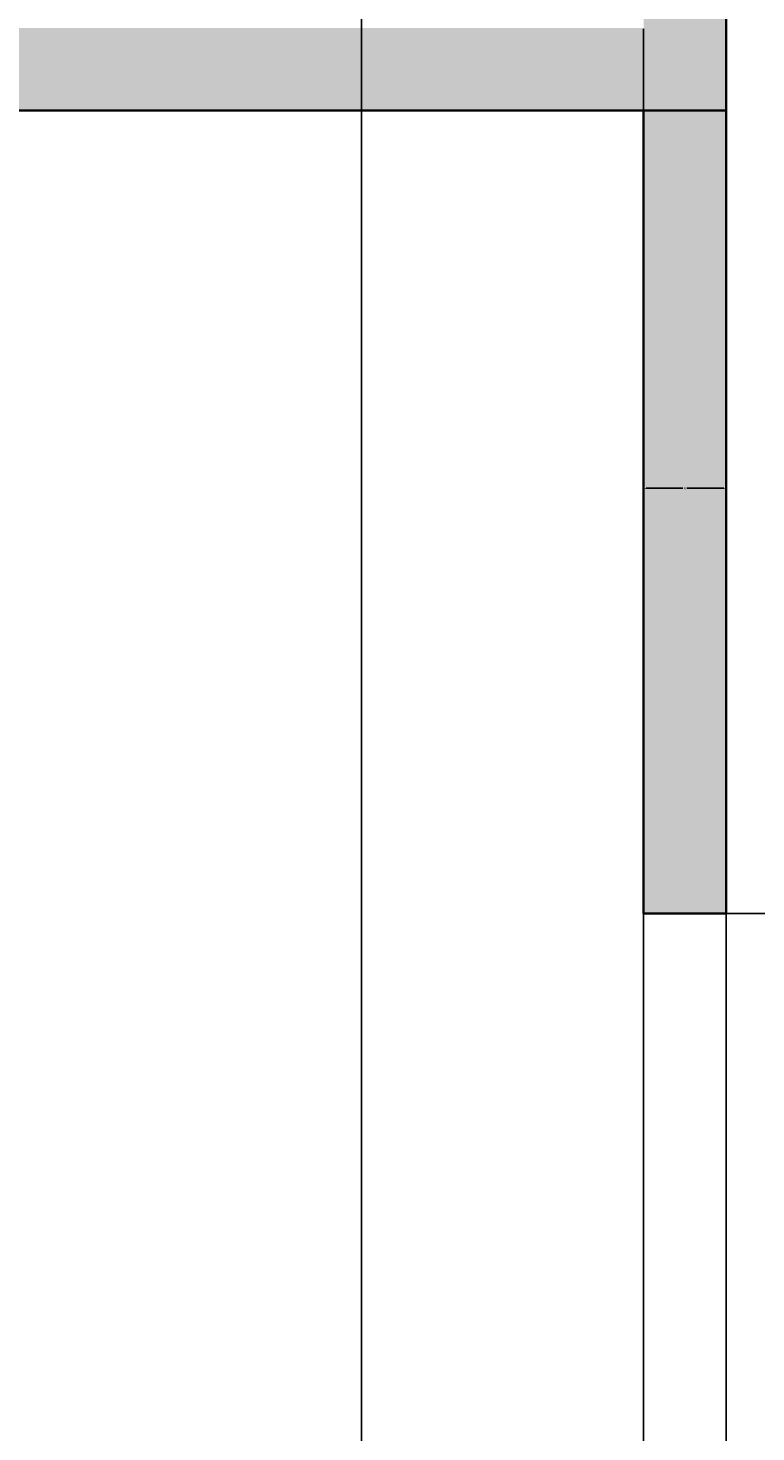
# Model space of a CAD drawing. Units: inches. Extents: x 2549 to 3108, y 1683 to 2362.
# Tile 16 of 30: x 2762 to 2815, y 1979 to 2081. Entities that reach past the tile are written whole.
import ezdxf

# ---------------------------------------------------------------- set-up
doc = ezdxf.new("R2010")
doc.units = ezdxf.units.IN
for name, color, linetype, lineweight in [('A-ANNO-DIMS', 2, 'Continuous', 18), ('A-WALL', 7, 'Continuous', 35), ('A-WALL-PATT', 89, 'Continuous', 13)]:
    doc.layers.add(name, color=color, linetype=linetype, lineweight=lineweight)
doc.layers.add('C-PKNG-VEHI-PATT', color=251, linetype='Continuous', lineweight=13, true_color=0x636466)
doc.layers.add('C-PVMT-PATT', color=9, linetype='Continuous', lineweight=13, true_color=0xc7c8ca)
doc.styles.get("Standard").update_dxf_attribs({"font": 'arial.ttf'})
doc.dimstyles.get("Standard").update_dxf_attribs({"dimtxt": 0.18, "dimasz": 0.18, "dimexe": 0.18, "dimexo": 0.0625, "dimgap": 0.09, "dimtad": 0, "dimtih": 1, "dimtoh": 1, "dimdec": 4, "dimzin": 0, "dimdsep": 46, "dimtxsty": 'Standard', "dimcen": 0.09, "dimadec": 0, "dimazin": 0, "dimtfac": 1, "dimtdec": 4, "dimtofl": 0, "dimtmove": 0, "dimatfit": 3, "dimfxl": 1, "dimtolj": 1, "dimtzin": 0, "dimarcsym": 0})

# ---------------------------------------------------------------- blocks, each defined once
blk = doc.blocks.new('*D43')
at = {"layer": 'A-ANNO-DIMS', "color": 0, "lineweight": -2, "transparency": 16777216}
for p, q in [((2734.64, 2080.46), (2734.64, 1683.44)), ((2806.64, 2080.46), (2806.64, 1683.44)), ((2734.82, 1683.62), (2770.43, 1683.62)), ((2806.46, 1683.62), (2770.86, 1683.62))]:
    blk.add_line(p, q, dxfattribs=at)
at = {"layer": 'A-ANNO-DIMS', "color": 0, "transparency": 16777216}
for points in [[(2734.82, 1683.65), (2734.82, 1683.59), (2734.64, 1683.62)], [(2806.46, 1683.65), (2806.46, 1683.59), (2806.64, 1683.62)]]:
    blk.add_solid(points, dxfattribs=at)
at = {"layer": 'Defpoints', "color": 0, "transparency": 16777216}
for p in [(2734.64, 2080.52), (2806.64, 2080.52), (2806.64, 1683.62)]:
    blk.add_point(p, dxfattribs=at)
at = {"layer": 'A-ANNO-DIMS', "color": 0, "transparency": 16777216, "insert": (2770.64, 1683.62), "char_height": 0.18, "attachment_point": 5}
blk.add_mtext('\\A1;72', dxfattribs=at)
blk = doc.blocks.new('*D44')
at = {"layer": 'A-ANNO-DIMS', "color": 0, "lineweight": -2, "transparency": 16777216}
for p, q in [((2662.64, 2040.99), (2662.64, 1683.44)), ((2806.64, 2016.13), (2806.64, 1683.44)), ((2662.82, 1683.62), (2734.36, 1683.62)), ((2806.46, 1683.62), (2734.92, 1683.62))]:
    blk.add_line(p, q, dxfattribs=at)
at = {"layer": 'A-ANNO-DIMS', "color": 0, "transparency": 16777216}
for points in [[(2662.82, 1683.65), (2662.82, 1683.59), (2662.64, 1683.62)], [(2806.46, 1683.65), (2806.46, 1683.59), (2806.64, 1683.62)]]:
    blk.add_solid(points, dxfattribs=at)
at = {"layer": 'Defpoints', "color": 0, "transparency": 16777216}
for p in [(2662.64, 2041.06), (2806.64, 2016.19), (2806.64, 1683.62)]:
    blk.add_point(p, dxfattribs=at)
at = {"layer": 'A-ANNO-DIMS', "color": 0, "transparency": 16777216, "insert": (2734.64, 1683.62), "char_height": 0.18, "attachment_point": 5}
blk.add_mtext('\\A1;144', dxfattribs=at)
blk = doc.blocks.new('*D46')
at = {"layer": 'A-ANNO-DIMS', "color": 0, "lineweight": -2, "transparency": 16777216}
for p, q in [((2812.64, 2140.46), (2812.64, 1683.44)), ((3034.64, 2134.46), (3034.64, 1683.44)), ((2812.82, 1683.62), (2923.35, 1683.62)), ((3034.46, 1683.62), (2923.93, 1683.62))]:
    blk.add_line(p, q, dxfattribs=at)
at = {"layer": 'A-ANNO-DIMS', "color": 0, "transparency": 16777216}
for points in [[(2812.82, 1683.65), (2812.82, 1683.59), (2812.64, 1683.62)], [(3034.46, 1683.65), (3034.46, 1683.59), (3034.64, 1683.62)]]:
    blk.add_solid(points, dxfattribs=at)
at = {"layer": 'Defpoints', "color": 0, "transparency": 16777216}
for p in [(2812.64, 2140.52), (3034.64, 2134.52), (3034.64, 1683.62)]:
    blk.add_point(p, dxfattribs=at)
at = {"layer": 'A-ANNO-DIMS', "color": 0, "transparency": 16777216, "insert": (2923.64, 1683.62), "char_height": 0.18, "attachment_point": 5}
blk.add_mtext('\\A1;222', dxfattribs=at)
blk = doc.blocks.new('*D47')
at = {"layer": 'A-ANNO-DIMS', "color": 0, "lineweight": -2, "transparency": 16777216}
for p, q in [((2806.64, 2016.25), (2806.64, 2047.27)), ((2812.64, 2016.25), (2812.64, 2047.27)), ((2806.82, 2047.09), (2809.49, 2047.09)), ((2812.46, 2047.09), (2809.79, 2047.09))]:
    blk.add_line(p, q, dxfattribs=at)
at = {"layer": 'A-ANNO-DIMS', "color": 0, "transparency": 16777216}
for points in [[(2806.82, 2047.12), (2806.82, 2047.06), (2806.64, 2047.09)], [(2812.46, 2047.12), (2812.46, 2047.06), (2812.64, 2047.09)]]:
    blk.add_solid(points, dxfattribs=at)
at = {"layer": 'Defpoints', "color": 0, "transparency": 16777216}
for p in [(2812.64, 2047.09), (2806.64, 2016.19), (2812.64, 2016.19)]:
    blk.add_point(p, dxfattribs=at)
at = {"layer": 'A-ANNO-DIMS', "color": 0, "transparency": 16777216, "insert": (2809.64, 2047.09), "char_height": 0.18, "attachment_point": 5}
blk.add_mtext('\\A1;6', dxfattribs=at)
blk = doc.blocks.new('*D48')
at = {"layer": 'A-ANNO-DIMS', "color": 0, "lineweight": -2, "transparency": 16777216}
for p, q in [((2812.71, 2016.19), (2843.72, 2016.19)), ((2843.54, 2016.01), (2843.54, 1981.04)), ((2843.54, 1945.7), (2843.54, 1980.68)), ((2812.71, 1945.52), (2843.72, 1945.52))]:
    blk.add_line(p, q, dxfattribs=at)
at = {"layer": 'A-ANNO-DIMS', "color": 0, "transparency": 16777216}
for points in [[(2843.51, 2016.01), (2843.57, 2016.01), (2843.54, 2016.19)], [(2843.51, 1945.7), (2843.57, 1945.7), (2843.54, 1945.52)]]:
    blk.add_solid(points, dxfattribs=at)
at = {"layer": 'Defpoints', "color": 0, "transparency": 16777216}
for p in [(2812.64, 2016.19), (2812.64, 1945.52), (2843.54, 1945.52)]:
    blk.add_point(p, dxfattribs=at)
at = {"layer": 'A-ANNO-DIMS', "color": 0, "transparency": 16777216, "insert": (2843.54, 1980.86), "char_height": 0.18, "attachment_point": 5}
blk.add_mtext('\\A1;70.67', dxfattribs=at)
blk = doc.blocks.new('*D52')
at = {"layer": 'A-ANNO-DIMS', "color": 0, "lineweight": -2, "transparency": 16777216}
for p, q in [((2812.64, 1891.59), (2812.64, 2362.32)), ((2872.64, 1891.59), (2872.64, 2362.32)), ((2812.82, 2362.14), (2842.42, 2362.14)), ((2872.46, 2362.14), (2842.86, 2362.14))]:
    blk.add_line(p, q, dxfattribs=at)
at = {"layer": 'A-ANNO-DIMS', "color": 0, "transparency": 16777216}
for points in [[(2812.82, 2362.17), (2812.82, 2362.11), (2812.64, 2362.14)], [(2872.46, 2362.17), (2872.46, 2362.11), (2872.64, 2362.14)]]:
    blk.add_solid(points, dxfattribs=at)
at = {"layer": 'Defpoints', "color": 0, "transparency": 16777216}
for p in [(2872.64, 2362.14), (2812.64, 1891.52), (2872.64, 1891.52)]:
    blk.add_point(p, dxfattribs=at)
at = {"layer": 'A-ANNO-DIMS', "color": 0, "transparency": 16777216, "insert": (2842.64, 2362.14), "char_height": 0.18, "attachment_point": 5}
blk.add_mtext('\\A1;60', dxfattribs=at)
blk = doc.blocks.new('*D59')
at = {"layer": 'A-ANNO-DIMS', "color": 0, "lineweight": -2, "transparency": 16777216}
for p, q in [((2680.98, 1761.59), (2680.98, 2362.32)), ((2786.16, 1761.59), (2786.16, 2362.32)), ((2681.16, 2362.14), (2733.11, 2362.14)), ((2785.98, 2362.14), (2734.02, 2362.14))]:
    blk.add_line(p, q, dxfattribs=at)
at = {"layer": 'A-ANNO-DIMS', "color": 0, "transparency": 16777216}
for points in [[(2681.16, 2362.17), (2681.16, 2362.11), (2680.98, 2362.14)], [(2785.98, 2362.17), (2785.98, 2362.11), (2786.16, 2362.14)]]:
    blk.add_solid(points, dxfattribs=at)
at = {"layer": 'Defpoints', "color": 0, "transparency": 16777216}
for p in [(2786.16, 2362.14), (2680.98, 1761.52), (2786.16, 1761.52)]:
    blk.add_point(p, dxfattribs=at)
at = {"layer": 'A-ANNO-DIMS', "color": 0, "transparency": 16777216, "insert": (2733.57, 2362.14), "char_height": 0.18, "attachment_point": 5}
blk.add_mtext('\\A1;105.18', dxfattribs=at)

msp = doc.modelspace()

# ---------------------------------------------------------------- hatches: boundary and pattern name
at = {"layer": 'A-WALL-PATT'}
h = msp.add_hatch(color=256, dxfattribs=at)
h.dxf.hatch_style = 1
h.paths.add_polyline_path([(2638.6427, 2272.5237), (3034.6427, 2272.5237), (3034.6427, 1936.5237), (3043.6427, 1936.5237), (3043.6427, 2281.5237), (2629.6427, 2281.5237), (2629.6427, 2074.5237), (2812.6427, 2074.5237), (2812.6427, 2140.5237), (2785.7177, 2140.5237), (2785.7177, 2134.5237), (2806.6427, 2134.5237), (2806.6427, 2080.5237), (2638.6427, 2080.5237)])
h.paths.add_polyline_path([(2638.6427, 1972.5237), (2662.6427, 1972.5237), (2662.6427, 2041.0557), (2653.6427, 2041.0557), (2653.6427, 1978.5237), (2629.6427, 1978.5237), (2629.6427, 1795.5237), (2662.6427, 1795.5237), (2881.6427, 1795.5237), (2881.6427, 1936.5237), (2965.9351, 1936.5237), (2965.9351, 1974.5439), (2959.9351, 1974.5439), (2959.9351, 1945.5237), (2881.6427, 1945.5237), (2872.6427, 1945.5237), (2872.6427, 1804.5237), (2662.6427, 1804.5237), (2638.6427, 1804.5237)])
h = msp.add_hatch(color=256, dxfattribs=at)
h.dxf.hatch_style = 1
h.paths.add_polyline_path([(2747.213, 2140.5237), (2638.6427, 2140.5237), (2638.6427, 2134.5237), (2747.213, 2134.5237)])
h.paths.add_polyline_path([(2734.6427, 2109.4935), (2728.6427, 2109.4935), (2728.6427, 2080.5237), (2734.6427, 2080.5237)])
h.paths.add_polyline_path([(2812.6427, 2074.5237), (2806.6427, 2074.5237), (2806.6427, 2016.1911), (2812.6427, 2016.1911)])
h.paths.add_polyline_path([(2812.6427, 1945.5237), (2806.6427, 1945.5237), (2806.6427, 1885.5237), (2872.6427, 1885.5237), (2872.6427, 1891.5237), (2812.6427, 1891.5237)])
h.paths.add_polyline_path([(2812.6427, 1855.9859), (2806.6427, 1855.9859), (2806.6427, 1804.5237), (2812.6427, 1804.5237)])
at = {"layer": 'C-PKNG-VEHI-PATT'}
h = msp.add_hatch(color=256, dxfattribs=at)
h.dxf.hatch_style = 1
edge = h.paths.add_edge_path()
edge.add_ellipse((2935.7258, 1791.964), major_axis=(-50.66, 0), ratio=0.84230387, start_angle=248.165046, end_angle=265.722579)
edge.add_line((2938.911, 1834.5507), (2925.8653, 1834.5507))
edge.add_ellipse((2929.0505, 1791.964), major_axis=(50.66, 0), ratio=0.84230387, start_angle=94.277421, end_angle=111.834954)
edge.add_line((2912.8508, 1832.3947), (2914.2044, 1822.2495))
edge.add_ellipse((2930.6538, 1783.1023), major_axis=(-49.3014, 0), ratio=0.84230387, start_angle=-85.12993, end_angle=-67.208085, ccw=False)
edge.add_line((2927.1247, 1824.5225), (2937.6516, 1824.5225))
edge.add_ellipse((2934.1225, 1783.1023), major_axis=(49.3014, 0), ratio=0.84230387, start_angle=67.208085, end_angle=85.12993, ccw=False)
edge.add_line((2950.5719, 1822.2495), (2951.9255, 1832.3947))
edge = h.paths.add_edge_path()
edge.add_ellipse((2903.4793, 1857.3351), major_axis=(-34.7979, 0), ratio=0.84230387, start_angle=180, end_angle=209.43857)
edge.add_ellipse((2961.297, 1857.3351), major_axis=(34.7979, 0), ratio=0.84230387, start_angle=150.56143, end_angle=180)
edge.add_line((2926.4991, 1857.3351), (2926.4991, 1843.7609))
edge.add_ellipse((2924.1251, 1844.3143), major_axis=(-0.2209, 3.9278), ratio=0.60383358, start_angle=89.002014, end_angle=253.657408, ccw=False)
edge.add_line((2921.7512, 1844.2222), (2921.7512, 1853.3975))
edge.add_line((2921.7512, 1853.3975), (2925.269, 1855.8484))
edge.add_ellipse((2925.4782, 1855.4931), major_axis=(0.4584, 0), ratio=0.84230387, start_angle=90, end_angle=134.480211, ccw=False)
edge.add_line((2925.4782, 1855.8792), (2926.4991, 1855.8792))
edge.add_line((2926.4991, 1855.8792), (2926.4991, 1857.3351))
edge.add_ellipse((2961.297, 1857.3351), major_axis=(34.7979, 0), ratio=0.84230387, start_angle=150.56143, end_angle=180, ccw=False)
edge.add_line((2932.3882, 1873.6501), (2932.3882, 1875.7801))
edge.add_ellipse((2932.3882, 1875.3939), major_axis=(0.4584, 0), ratio=0.84230387, start_angle=90, end_angle=127.93313)
edge.add_line((2932.1366, 1875.7167), (2928.5915, 1873.7564))
edge.add_ellipse((2899.9271, 2002.4692), major_axis=(155.4756, 0), ratio=0.84230387, start_angle=-80.743434, end_angle=-77.445067, ccw=False)
edge.add_ellipse((2949.4402, 1715.2151), major_axis=(-189.1422, 0), ratio=0.84230387, start_angle=-79.790461, end_angle=-77.555373)
edge.add_ellipse((3300.3614, 1852.5642), major_axis=(-386.1662, 0), ratio=0.84230387, start_angle=-2.863715, end_angle=2.198541)
edge.add_ellipse((2929.0505, 1792.5159), major_axis=(-55.6192, 0), ratio=0.84230387, start_angle=-85.917589, end_angle=-72.280047, ccw=False)
edge.add_line((2925.7129, 1839.2798), (2939.0634, 1839.2798))
edge.add_ellipse((2935.7258, 1792.5159), major_axis=(55.6192, 0), ratio=0.84230387, start_angle=72.280047, end_angle=85.917589, ccw=False)
edge.add_ellipse((2564.4149, 1852.5642), major_axis=(-386.1662, 0), ratio=0.84230387, start_angle=177.801459, end_angle=182.863715)
edge.add_ellipse((2915.3361, 1715.2151), major_axis=(189.1422, 0), ratio=0.84230387, start_angle=77.555373, end_angle=79.790461)
edge.add_ellipse((2964.8492, 2002.4692), major_axis=(-155.4756, 0), ratio=0.84230387, start_angle=77.445067, end_angle=80.743434, ccw=False)
edge.add_line((2936.1848, 1873.7564), (2932.6397, 1875.7167))
edge.add_ellipse((2932.3882, 1875.3939), major_axis=(0.4584, 0), ratio=0.84230387, start_angle=52.06687, end_angle=90)
edge.add_line((2932.3882, 1875.7801), (2932.3882, 1873.6501))
edge.add_ellipse((2903.4793, 1857.3351), major_axis=(-34.7979, 0), ratio=0.84230387, start_angle=180, end_angle=209.43857, ccw=False)
edge.add_line((2938.2772, 1857.3351), (2938.2772, 1855.8792))
edge.add_line((2938.2772, 1855.8792), (2939.4059, 1855.8792))
edge.add_ellipse((2939.2981, 1855.4931), major_axis=(-0.4584, 0), ratio=0.84230387, start_angle=225.519789, end_angle=270, ccw=False)
edge.add_line((2939.5903, 1855.7906), (2943.0251, 1853.3975))
edge.add_line((2943.0251, 1853.3975), (2943.0251, 1844.2222))
edge.add_ellipse((2940.6512, 1844.3143), major_axis=(0.2209, 3.9278), ratio=0.60383358, start_angle=106.342592, end_angle=270.997986, ccw=False)
edge.add_line((2938.2772, 1843.7609), (2938.2772, 1857.3351))
edge = h.paths.add_edge_path()
edge.add_ellipse((2932.3882, 1865.1973), major_axis=(91.081, 0), ratio=0.84230387, start_angle=256.401865, end_angle=283.598135, ccw=False)
edge.add_line((2914.2044, 1790.0239), (2914.2044, 1778.3622))
edge.add_ellipse((2932.3882, 1853.5356), major_axis=(91.081, 0), ratio=0.84230387, start_angle=256.401865, end_angle=283.598135)
edge.add_line((2950.5719, 1778.3622), (2950.5719, 1790.0239))
edge = h.paths.add_edge_path()
edge.add_ellipse((2948.7383, 1772.3145), major_axis=(1.8336, 0), ratio=0.84230387, start_angle=0, end_angle=90)
edge.add_line((2948.7383, 1773.859), (2916.038, 1773.859))
edge.add_ellipse((2916.038, 1772.3145), major_axis=(1.8336, 0), ratio=0.84230387, start_angle=90, end_angle=180)
edge.add_line((2914.2044, 1772.3145), (2914.2044, 1760.2558))
edge.add_line((2914.2044, 1760.2558), (2950.5719, 1760.2558))
edge.add_line((2950.5719, 1760.2558), (2950.5719, 1772.3145))
h.paths.add_polyline_path([(2748.8496, 2101.6383), (2798.148, 2101.6383), (2798.148, 2111.4248), (2748.8496, 2111.4248)], flags=9)
h.paths.add_polyline_path([(2685.2081, 2101.489), (2719.3253, 2101.489), (2719.3253, 2111.2819), (2685.2081, 2111.2819)], flags=9)
h.paths.add_polyline_path([(2814.6852, 1907.1328), (2847.8384, 1907.1328), (2847.8384, 1916.9258), (2814.6852, 1916.9258)], flags=9)
h.paths.add_polyline_path([(2814.3906, 1835.5864), (2848.0172, 1835.5864), (2848.0172, 1845.3794), (2814.3906, 1845.3794)], flags=9)
h.paths.add_polyline_path([(2800.5245, 1759.1674), (2853.7435, 1759.1674), (2853.7435, 1768.954), (2800.5245, 1768.954)], flags=9)
h.paths.add_polyline_path([(2972.4611, 1807.3305), (3015.3943, 1807.3305), (3015.3943, 1817.117), (2972.4611, 1817.117)], flags=9)
h.paths.add_polyline_path([(2902.3327, 1888.6731), (2937.9131, 1888.6731), (2937.9131, 1898.4661), (2902.3327, 1898.4661)], flags=9)
h.paths.add_polyline_path([(2712.1779, 1878.9039), (2754.1257, 1878.9039), (2754.1257, 1888.6904), (2712.1779, 1888.6904)], flags=9)
h.paths.add_polyline_path([(2614.0056, 2012.812), (2650.0251, 2012.812), (2650.0251, 2022.4371), (2614.0056, 2022.4371)], flags=9)
h.paths.add_polyline_path([(2713.3129, 2003.1645), (2747.4237, 2003.1645), (2747.4237, 2012.951), (2713.3129, 2012.951)], flags=9)
h.paths.add_polyline_path([(2950.1379, 2001.6934), (2982.2992, 2001.6934), (2982.2992, 2011.48), (2950.1379, 2011.48)], flags=9)
h.paths.add_polyline_path([(2940.864, 2238.5537), (2997.5066, 2238.5537), (2997.5066, 2248.3466), (2940.864, 2248.3466)], flags=9)
h.paths.add_polyline_path([(2821.5457, 2202.8348), (2855.663, 2202.8348), (2855.663, 2212.6278), (2821.5457, 2212.6278)], flags=9)
h.paths.add_polyline_path([(2661.8026, 2238.6249), (2718.4451, 2238.6249), (2718.4451, 2248.4179), (2661.8026, 2248.4179)], flags=9)
at = {"layer": 'C-PVMT-PATT'}
h = msp.add_hatch(color=256, dxfattribs=at)
h.dxf.hatch_style = 1
h.paths.add_polyline_path([(3067.6427, 2305.5237), (2605.6427, 2305.5237), (2605.6427, 2074.5237), (2629.6427, 2074.5237), (2629.6427, 2281.5237), (3043.6427, 2281.5237), (3043.6427, 1885.5237), (3043.6427, 1872.8745), (3031.1672, 1872.8745), (3031.1672, 1862.5731), (2995.8054, 1862.5731), (2995.8054, 1872.8745), (2983.1752, 1872.8745), (2983.1752, 1885.5237), (2881.6427, 1885.5237), (2881.6427, 1795.5237), (2751.0977, 1795.5237), (2751.0977, 1761.5237), (2786.1577, 1761.5237), (2786.1577, 1723.5237), (2881.84, 1723.5237), (2881.84, 1714.5237), (3067.6427, 1714.5237), (3067.6427, 1723.5237)])
edge = h.paths.add_edge_path(flags=16)
edge.add_ellipse((2949.4402, 1710.9683), major_axis=(-194.1014, 0), ratio=0.84230387, start_angle=-77.874034, end_angle=-76.219471, ccw=False)
edge.add_ellipse((2949.4402, 1715.2151), major_axis=(-189.1422, 0), ratio=0.84230387, start_angle=-79.790461, end_angle=-77.555373, ccw=False)
edge.add_ellipse((2899.9271, 2002.4692), major_axis=(155.4756, 0), ratio=0.84230387, start_angle=-80.743434, end_angle=-77.445067)
edge.add_line((2928.5915, 1873.7564), (2932.3882, 1875.8558))
edge.add_line((2932.3882, 1875.8558), (2936.1848, 1873.7564))
edge.add_ellipse((2964.8492, 2002.4692), major_axis=(-155.4756, 0), ratio=0.84230387, start_angle=77.445067, end_angle=80.743434)
edge.add_ellipse((2915.3361, 1715.2151), major_axis=(189.1422, 0), ratio=0.84230387, start_angle=77.555373, end_angle=79.790461, ccw=False)
edge.add_ellipse((2915.3361, 1710.9683), major_axis=(-194.1014, 0), ratio=0.84230387, start_angle=256.219471, end_angle=257.874034, ccw=False)
edge.add_ellipse((2628.2871, 1850.2612), major_axis=(-327.2532, 0), ratio=0.84230387, start_angle=182.17995, end_angle=183.650428, ccw=False)
edge.add_ellipse((2955.5637, 1861.9334), major_axis=(-0.9168, 0), ratio=0.84230387, start_angle=180, end_angle=270, ccw=False)
edge.add_line((2956.4805, 1862.3857), (2956.4805, 1846.4866))
edge.add_ellipse((2955.5637, 1846.939), major_axis=(-0.9168, 0), ratio=0.84230387, start_angle=90, end_angle=180, ccw=False)
edge.add_ellipse((-3607.0606, 1835.832), major_axis=(-6562.6242, 0), ratio=0.84230387, start_angle=179.61613322, end_angle=180.09022909, ccw=False)
edge.add_ellipse((2955.5637, 1791.0926), major_axis=(0.9168, 0), ratio=0.84230387, start_angle=0, end_angle=90, ccw=False)
edge.add_line((2956.4805, 1791.545), (2956.4805, 1775.6459))
edge.add_ellipse((2955.5637, 1776.0982), major_axis=(0.9168, 0), ratio=0.84230387, start_angle=270, end_angle=360, ccw=False)
edge.add_ellipse((-3607.0606, 1835.832), major_axis=(-6562.6242, 0), ratio=0.84230387, start_angle=179.3813568, end_angle=179.47172853, ccw=False)
edge.add_ellipse((2954.5907, 1763.8768), major_axis=(-1.3752, 0), ratio=0.84230387, start_angle=179.371763, end_angle=248.464757, ccw=False)
edge.add_ellipse((-3607.519, 1835.832), major_axis=(-6564.0409, 0), ratio=0.842303863, start_angle=179.35344594, end_angle=179.37176282, ccw=False)
edge.add_ellipse((2952.6829, 1761.8002), major_axis=(3.2503, 0), ratio=0.84230387, start_angle=-90, end_angle=-0.646554, ccw=False)
edge.add_line((2952.6829, 1759.0625), (2912.0934, 1759.0625))
edge.add_ellipse((2912.0934, 1761.8002), major_axis=(3.2503, 0), ratio=0.84230387, start_angle=180.646554, end_angle=270, ccw=False)
edge.add_ellipse((9472.2953, 1835.832), major_axis=(-6564.0409, 0), ratio=0.842303871, start_angle=0.62823722, end_angle=0.6465541, ccw=False)
edge.add_ellipse((2910.1856, 1763.8768), major_axis=(1.3752, 0), ratio=0.84230387, start_angle=111.535244, end_angle=180.628237, ccw=False)
edge.add_ellipse((9471.8369, 1835.832), major_axis=(-6562.6242, 0), ratio=0.84230387, start_angle=0.52827147, end_angle=0.6465541, ccw=False)
edge.add_ellipse((2909.2126, 1776.0982), major_axis=(-0.9168, 0), ratio=0.84230387, start_angle=0, end_angle=90, ccw=False)
edge.add_line((2908.2958, 1775.6459), (2908.2958, 1791.545))
edge.add_ellipse((2909.2126, 1791.0926), major_axis=(-0.9168, 0), ratio=0.84230387, start_angle=-90, end_angle=0, ccw=False)
edge.add_ellipse((9471.8369, 1835.832), major_axis=(-6562.6242, 0), ratio=0.84230387, start_angle=-0.09022909, end_angle=0.38386678, ccw=False)
edge.add_ellipse((2909.2126, 1846.939), major_axis=(-0.9168, 0), ratio=0.84230387, start_angle=0, end_angle=90, ccw=False)
edge.add_line((2908.2958, 1846.4866), (2908.2958, 1862.3857))
edge.add_ellipse((2909.2126, 1861.9334), major_axis=(0.9168, 0), ratio=0.84230387, start_angle=90, end_angle=180, ccw=False)
edge.add_ellipse((3236.4892, 1850.2612), major_axis=(327.2532, 0), ratio=0.84230387, start_angle=176.349572, end_angle=177.82005, ccw=False)
edge = h.paths.add_edge_path(flags=0)
edge.add_ellipse((2903.4793, 1857.3351), major_axis=(-34.7979, 0), ratio=0.84230387, start_angle=180, end_angle=209.43857, ccw=False)
edge.add_line((2938.2772, 1857.3351), (2938.2772, 1855.8792))
edge.add_line((2938.2772, 1855.8792), (2939.4631, 1855.8792))
edge.add_line((2939.4631, 1855.8792), (2943.0251, 1853.3975))
edge.add_line((2943.0251, 1853.3975), (2943.0251, 1844.2222))
edge.add_ellipse((2940.6512, 1844.3143), major_axis=(0.2209, 3.9278), ratio=0.60383358, start_angle=106.342592, end_angle=270.997986, ccw=False)
edge.add_line((2938.2772, 1843.7609), (2938.2772, 1857.3351))
edge.add_ellipse((2903.4793, 1857.3351), major_axis=(-34.7979, 0), ratio=0.84230387, start_angle=180, end_angle=209.43857)
edge.add_ellipse((2961.297, 1857.3351), major_axis=(34.7979, 0), ratio=0.84230387, start_angle=150.56143, end_angle=180)
edge.add_line((2926.4991, 1857.3351), (2926.4991, 1843.7609))
edge.add_ellipse((2924.1251, 1844.3143), major_axis=(-0.2209, 3.9278), ratio=0.60383358, start_angle=89.002014, end_angle=253.657408, ccw=False)
edge.add_line((2921.7512, 1844.2222), (2921.7512, 1853.3975))
edge.add_line((2921.7512, 1853.3975), (2925.3132, 1855.8792))
edge.add_line((2925.3132, 1855.8792), (2926.4991, 1855.8792))
edge.add_line((2926.4991, 1855.8792), (2926.4991, 1857.3351))
edge.add_ellipse((2961.297, 1857.3351), major_axis=(34.7979, 0), ratio=0.84230387, start_angle=150.56143, end_angle=180, ccw=False)
edge = h.paths.add_edge_path(flags=0)
edge.add_ellipse((2929.0505, 1791.964), major_axis=(50.66, 0), ratio=0.84230387, start_angle=94.277421, end_angle=111.834954, ccw=False)
edge.add_line((2925.8653, 1834.5507), (2938.911, 1834.5507))
edge.add_ellipse((2935.7258, 1791.964), major_axis=(-50.66, 0), ratio=0.84230387, start_angle=248.165046, end_angle=265.722579, ccw=False)
edge.add_line((2951.9255, 1832.3947), (2950.5719, 1822.2495))
edge.add_ellipse((2934.1225, 1783.1023), major_axis=(49.3014, 0), ratio=0.84230387, start_angle=67.208085, end_angle=85.12993)
edge.add_line((2937.6516, 1824.5225), (2927.1247, 1824.5225))
edge.add_ellipse((2930.6538, 1783.1023), major_axis=(-49.3014, 0), ratio=0.84230387, start_angle=-85.12993, end_angle=-67.208085)
edge.add_line((2914.2044, 1822.2495), (2912.8508, 1832.3947))
edge = h.paths.add_edge_path(flags=0)
edge.add_line((2910.1338, 1829.4651), (2912.6432, 1821.2711))
edge.add_ellipse((5203.7787, 1816.4367), major_axis=(-2291.1426, 0), ratio=0.84230387, start_angle=-0.1208974, end_angle=0.3640763)
edge.add_line((2912.7012, 1801.8782), (2910.3305, 1792.5698))
edge.add_ellipse((9471.8369, 1835.832), major_axis=(-6561.7074, 0), ratio=0.84230387, start_angle=0.05559431, end_angle=0.37776419, ccw=False)
edge = h.paths.add_edge_path(flags=0)
edge.add_ellipse((-3607.0606, 1835.832), major_axis=(6561.7074, 0), ratio=0.84230387, start_angle=-0.37776419, end_angle=-0.05559431, ccw=False)
edge.add_line((2954.4458, 1792.5698), (2952.0751, 1801.8782))
edge.add_ellipse((660.9976, 1816.4367), major_axis=(2291.1426, 0), ratio=0.84230387, start_angle=-0.3640763, end_angle=0.1208974)
edge.add_line((2952.1331, 1821.2711), (2954.6425, 1829.4651))
edge = h.paths.add_edge_path(flags=0)
edge.add_ellipse((2932.3882, 1865.1973), major_axis=(91.081, 0), ratio=0.84230387, start_angle=256.401865, end_angle=283.598135)
edge.add_line((2950.5719, 1790.0239), (2950.5719, 1778.3622))
edge.add_ellipse((2932.3882, 1853.5356), major_axis=(91.081, 0), ratio=0.84230387, start_angle=256.401865, end_angle=283.598135, ccw=False)
edge.add_line((2914.2044, 1778.3622), (2914.2044, 1790.0239))
edge = h.paths.add_edge_path(flags=0)
edge.add_line((2916.038, 1773.859), (2948.7383, 1773.859))
edge.add_ellipse((2948.7383, 1772.3145), major_axis=(1.8336, 0), ratio=0.84230387, start_angle=0, end_angle=90, ccw=False)
edge.add_line((2950.5719, 1772.3145), (2950.5719, 1760.2558))
edge.add_line((2950.5719, 1760.2558), (2914.2044, 1760.2558))
edge.add_line((2914.2044, 1760.2558), (2914.2044, 1772.3145))
edge.add_ellipse((2916.038, 1772.3145), major_axis=(1.8336, 0), ratio=0.84230387, start_angle=90, end_angle=180, ccw=False)
h.paths.add_polyline_path([(2629.6427, 1978.5237), (2605.6427, 1978.5237), (2605.6427, 1723.5237), (2629.6427, 1723.5237), (2629.6427, 1795.5237)], flags=17)
h.paths.add_polyline_path([(2800.5245, 1759.1674), (2853.7435, 1759.1674), (2853.7435, 1768.954), (2800.5245, 1768.954)], flags=24)
h.paths.add_polyline_path([(2972.4611, 1807.3305), (3015.3943, 1807.3305), (3015.3943, 1817.117), (2972.4611, 1817.117)], flags=24)

# ---------------------------------------------------------------- linework, layer by layer
at = {"layer": 'A-WALL'}
for p, q in [((2812.6427, 2074.5237), (2812.6427, 2140.5237)), ((2629.6427, 2074.5237), (2812.6427, 2074.5237)), ((2806.6427, 2074.5237), (2806.6427, 2016.1911)), ((2812.6427, 2074.5237), (2812.6427, 2016.1911)), ((2806.6427, 2016.1911), (2812.6427, 2016.1911))]:
    msp.add_line(p, q, dxfattribs=at)

# ---------------------------------------------------------------- dimensions: what is measured, and where the dimension line sits
at = {"layer": 'A-ANNO-DIMS'}
for base, p1, p2, override, picture, middle in [((2786.1577, 2362.1425), (2680.9778, 1761.5237), (2786.1577, 1761.5237), {"dimdec": 2, "dimlfac": 1, "dimrnd": 0, "dimzin": 0, "dimdsep": 46, "dimlunit": 2}, '*D59', (2733.5678, 2362.1425)), ((2872.6427, 2362.1425), (2812.6427, 1891.5237), (2872.6427, 1891.5237), {"dimdec": 0, "dimlfac": 1, "dimrnd": 0, "dimzin": 0, "dimdsep": 46, "dimlunit": 2}, '*D52', (2842.6427, 2362.1425)), ((3034.6427, 1683.6237), (2812.6427, 2140.5237), (3034.6427, 2134.5237), {"dimdec": 0, "dimlfac": 1, "dimrnd": 0, "dimzin": 0, "dimdsep": 46, "dimlunit": 2}, '*D46', (2923.6427, 1683.6237)), ((2806.6427, 1683.6237), (2734.6427, 2080.5237), (2806.6427, 2080.5237), {"dimdec": 0, "dimlfac": 1, "dimrnd": 0, "dimzin": 0, "dimdsep": 46, "dimlunit": 2}, '*D43', (2770.6427, 1683.6237)), ((2812.6427, 2047.0911), (2806.6427, 2016.1911), (2812.6427, 2016.1911), {"dimdec": 0, "dimlfac": 1, "dimrnd": 0, "dimzin": 0, "dimdsep": 46, "dimlunit": 2}, '*D47', (2809.6427, 2047.0911)), ((2806.6427, 1683.6237), (2662.6427, 2041.0557), (2806.6427, 2016.1911), {"dimdec": 0, "dimlfac": 1, "dimrnd": 0, "dimzin": 0, "dimdsep": 46, "dimlunit": 2}, '*D44', (2734.6427, 1683.6237))]:
    dim = msp.add_linear_dim(base=base, p1=p1, p2=p2, dimstyle='Standard', override=override, dxfattribs=at)
    dim.commit()
    dim.dimension.update_dxf_attribs({"geometry": picture, "text_midpoint": middle})
dim = msp.add_linear_dim(base=(2843.5427, 1945.5237), p1=(2812.6427, 2016.1911), p2=(2812.6427, 1945.5237), angle=270, dimstyle='Standard', override={"dimdec": 2, "dimlfac": 1, "dimrnd": 0, "dimzin": 0, "dimdsep": 46, "dimlunit": 2}, dxfattribs=at)
dim.commit()
dim.dimension.update_dxf_attribs({"geometry": '*D48', "text_midpoint": (2843.5427, 1980.8574)})

doc.saveas('drawing.dxf')
